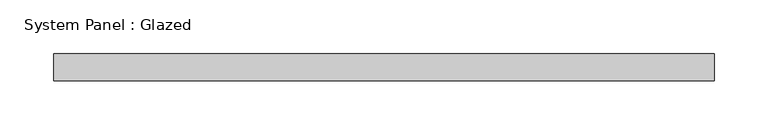
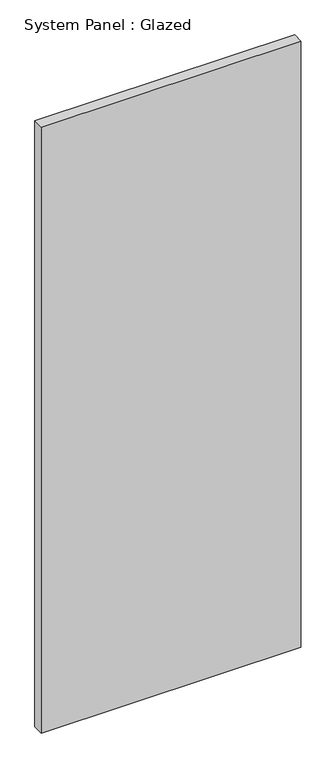
"""IFC4 building model written with IfcOpenShell, lengths in millimetres: plate geometry, System Panel : Glazed."""

from ifc_helpers import new_model, si_unit, origin, origin_with_axes, place, context, project, spatial, polyline, outline, extrude, source, transform, mapped, element, save


def system_panel_glazed_c72e3a3f(model_context):
    return source(origin(), model_context, "Body", "SweptSolid", [
        extrude(outline(polyline([(307.975, 19.05), (-307.975, 19.05), (-307.975, 44.45), (307.975, 44.45), (307.975, 19.05)])), origin_with_axes(), (0.0, 0.0, 1.0), 1518.4701172),
    ])


if __name__ == "__main__":
    model = new_model("IFC4")
    model_context = context("Model", 3, world=origin())
    ifc_project = project(units=[si_unit("LENGTHUNIT", "METRE", prefix="MILLI")], contexts=[model_context])
    site = spatial("IfcSite", under=ifc_project)
    building = spatial("IfcBuilding", under=site)
    placement = place(None, origin())
    system_panel_glazed_shape = system_panel_glazed_c72e3a3f(model_context)
    element("IfcPlate", 1, ObjectType="System Panel : Glazed", at=placement, inside=building, context=model_context, shape_type="MappedRepresentation", body=[
        mapped(system_panel_glazed_shape, transform((0.0, 0.0, 0.0), x_axis=(1.0, 0.0, 0.0), y_axis=(0.0, 1.0, 0.0), z_axis=(0.0, 0.0, 1.0))),
    ])
    save(model, "model.ifc")

# Revit data of these elements
# Type "System Panel : Glazed"
#   Construction Type Id = "GSP4R"
#   Analytic Construction = "1/8 in Pilkington single glazing"
#   Visual Light Transmittance = 0.9
#   Solar Heat Gain Coefficient = 0.86
#   Heat Transfer Coefficient (U) = 1.18115 BTU/(h·ft²·°F)
#   Define Thermal Properties by = 1
# Element 1 (IfcPlate, "System Panel : Glazed")
#   Materials on its faces: "Glass"
# Materials
#   "Glass": class "Glass", colour RGB 0 128 192, transparency 0.75, Description = "Soda Lime Glass", Cost = 0
